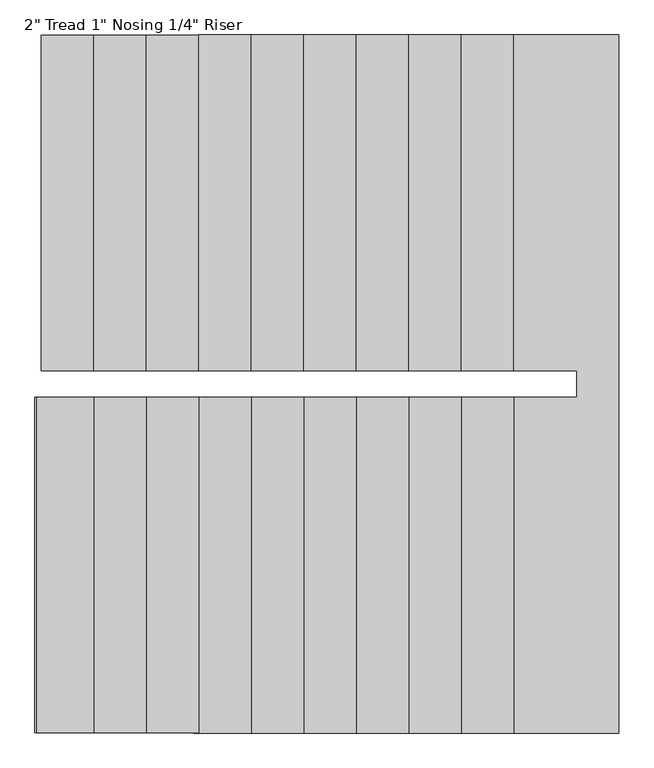
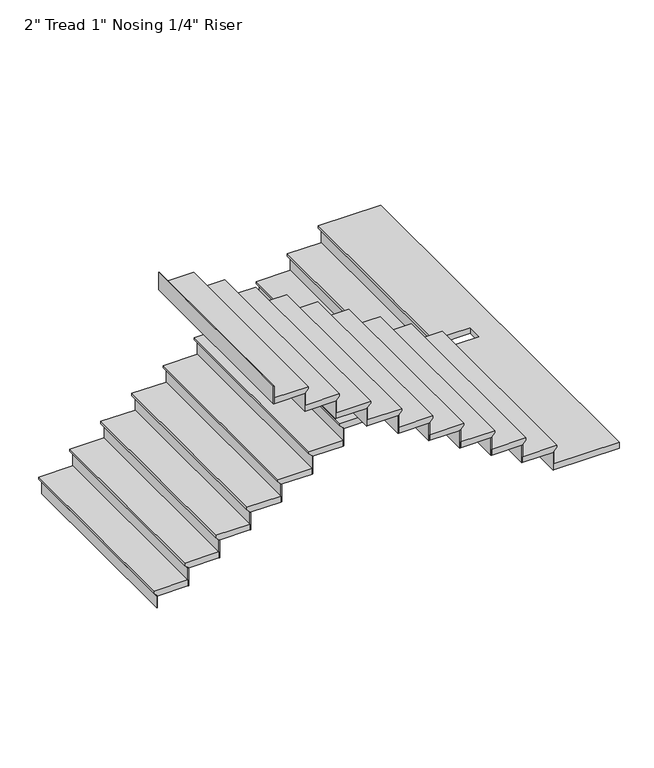
"""IFC4 building model written with IfcOpenShell, lengths in millimetres: stair flight geometry."""

from ifc_helpers import new_model, si_unit, origin, place, context, project, spatial, faceted_brep, source, transform, mapped, element, save


def stair_flight_de280899(model_context):
    return source(origin(), model_context, "Body", "Brep", [
        faceted_brep([(-6414.1711241, 10106.9344295, 3181.35), (-6414.1711241, 10106.9344295, 3200.4), (-6414.1711241, 11732.5344295, 3200.4), (-6414.1711241, 11732.5344295, 3181.35), (-6388.7711241, 10106.9344295, 3155.95), (-6388.7711241, 11732.5344295, 3155.95), (-6134.7711241, 10106.9344295, 3200.4), (-6134.7711241, 11732.5344295, 3200.4), (-6388.7711241, 11732.5344295, 3149.6), (-6134.7711241, 11732.5344295, 3149.6), (-6134.7711241, 10106.9344295, 3149.6), (-6388.7711241, 10106.9344295, 3149.6)], [[[0, 1, 2, 3]], [[4, 0, 3, 5]], [[2, 1, 6, 7]], [[8, 9, 10, 11]], [[2, 7, 9, 8, 5, 3]], [[8, 11, 4, 5]], [[6, 1, 0, 4, 11, 10]], [[7, 6, 10, 9]]]),
        faceted_brep([(-6388.7711241, 10106.9344295, 3149.6), (-6388.7711241, 10106.9344295, 3048.0), (-6382.4211241, 10106.9344295, 3048.0), (-6382.4211241, 10106.9344295, 3149.6), (-6388.7711241, 11732.5344295, 3149.6), (-6382.4211241, 11732.5344295, 3149.6), (-6382.4211241, 11732.5344295, 3048.0), (-6388.7711241, 11732.5344295, 3048.0)], [[[0, 1, 2, 3]], [[4, 5, 6, 7]], [[1, 0, 4, 7]], [[2, 1, 7, 6]], [[3, 2, 6, 5]], [[0, 3, 5, 4]]]),
        faceted_brep([(-6134.7711241, 10106.9344295, 3302.0), (-6134.7711241, 10106.9344295, 3149.6), (-6128.4211241, 10106.9344295, 3149.6), (-6128.4211241, 10106.9344295, 3302.0), (-6134.7711241, 11732.5344295, 3302.0), (-6128.4211241, 11732.5344295, 3302.0), (-6128.4211241, 11732.5344295, 3149.6), (-6134.7711241, 11732.5344295, 3149.6)], [[[0, 1, 2, 3]], [[4, 5, 6, 7]], [[1, 0, 4, 7]], [[2, 1, 7, 6]], [[3, 2, 6, 5]], [[0, 3, 5, 4]]]),
        faceted_brep([(-6160.1711241, 11732.5344295, 3352.8), (-6160.1711241, 10106.9344295, 3352.8), (-5880.7711241, 10106.9344295, 3352.8), (-5880.7711241, 11732.5344295, 3352.8), (-6134.7711241, 11732.5344295, 3302.0), (-5880.7711241, 11732.5344295, 3302.0), (-5880.7711241, 10106.9344295, 3302.0), (-6134.7711241, 10106.9344295, 3302.0), (-6134.7711241, 11732.5344295, 3308.35), (-6160.1711241, 11732.5344295, 3333.75), (-6134.7711241, 10106.9344295, 3308.35), (-6160.1711241, 10106.9344295, 3333.75)], [[[0, 1, 2, 3]], [[4, 5, 6, 7]], [[0, 3, 5, 4, 8, 9]], [[4, 7, 10, 8]], [[2, 1, 11, 10, 7, 6]], [[3, 2, 6, 5]], [[11, 1, 0, 9]], [[10, 11, 9, 8]]]),
        faceted_brep([(-5880.7711241, 10106.9344295, 3454.4), (-5880.7711241, 10106.9344295, 3302.0), (-5874.4211241, 10106.9344295, 3302.0), (-5874.4211241, 10106.9344295, 3454.4), (-5880.7711241, 11732.5344295, 3454.4), (-5874.4211241, 11732.5344295, 3454.4), (-5874.4211241, 11732.5344295, 3302.0), (-5880.7711241, 11732.5344295, 3302.0)], [[[0, 1, 2, 3]], [[4, 5, 6, 7]], [[1, 0, 4, 7]], [[2, 1, 7, 6]], [[3, 2, 6, 5]], [[0, 3, 5, 4]]]),
        faceted_brep([(-5906.1711241, 11732.5344295, 3505.2), (-5906.1711241, 10106.9344295, 3505.2), (-5626.7711241, 10106.9344295, 3505.2), (-5626.7711241, 11732.5344295, 3505.2), (-5880.7711241, 11732.5344295, 3454.4), (-5626.7711241, 11732.5344295, 3454.4), (-5626.7711241, 10106.9344295, 3454.4), (-5880.7711241, 10106.9344295, 3454.4), (-5880.7711241, 11732.5344295, 3460.75), (-5906.1711241, 11732.5344295, 3486.15), (-5880.7711241, 10106.9344295, 3460.75), (-5906.1711241, 10106.9344295, 3486.15)], [[[0, 1, 2, 3]], [[4, 5, 6, 7]], [[0, 3, 5, 4, 8, 9]], [[4, 7, 10, 8]], [[2, 1, 11, 10, 7, 6]], [[3, 2, 6, 5]], [[11, 1, 0, 9]], [[10, 11, 9, 8]]]),
        faceted_brep([(-5626.7711241, 10106.9344295, 3606.8), (-5626.7711241, 10106.9344295, 3454.4), (-5620.4211241, 10106.9344295, 3454.4), (-5620.4211241, 10106.9344295, 3606.8), (-5626.7711241, 11732.5344295, 3606.8), (-5620.4211241, 11732.5344295, 3606.8), (-5620.4211241, 11732.5344295, 3454.4), (-5626.7711241, 11732.5344295, 3454.4)], [[[0, 1, 2, 3]], [[4, 5, 6, 7]], [[1, 0, 4, 7]], [[2, 1, 7, 6]], [[3, 2, 6, 5]], [[0, 3, 5, 4]]]),
        faceted_brep([(-5652.1711241, 11732.5344295, 3657.6), (-5652.1711241, 10106.9344295, 3657.6), (-5372.7711241, 10106.9344295, 3657.6), (-5372.7711241, 11732.5344295, 3657.6), (-5626.7711241, 11732.5344295, 3606.8), (-5372.7711241, 11732.5344295, 3606.8), (-5372.7711241, 10106.9344295, 3606.8), (-5626.7711241, 10106.9344295, 3606.8), (-5626.7711241, 11732.5344295, 3613.15), (-5652.1711241, 11732.5344295, 3638.55), (-5626.7711241, 10106.9344295, 3613.15), (-5652.1711241, 10106.9344295, 3638.55)], [[[0, 1, 2, 3]], [[4, 5, 6, 7]], [[0, 3, 5, 4, 8, 9]], [[4, 7, 10, 8]], [[2, 1, 11, 10, 7, 6]], [[3, 2, 6, 5]], [[11, 1, 0, 9]], [[10, 11, 9, 8]]]),
        faceted_brep([(-5372.7711241, 10106.9344295, 3759.2), (-5372.7711241, 10106.9344295, 3606.8), (-5366.4211241, 10106.9344295, 3606.8), (-5366.4211241, 10106.9344295, 3759.2), (-5372.7711241, 11732.5344295, 3759.2), (-5366.4211241, 11732.5344295, 3759.2), (-5366.4211241, 11732.5344295, 3606.8), (-5372.7711241, 11732.5344295, 3606.8)], [[[0, 1, 2, 3]], [[4, 5, 6, 7]], [[1, 0, 4, 7]], [[2, 1, 7, 6]], [[3, 2, 6, 5]], [[0, 3, 5, 4]]]),
        faceted_brep([(-5398.1711241, 11732.5344295, 3810.0), (-5398.1711241, 10106.9344295, 3810.0), (-5118.7711241, 10106.9344295, 3810.0), (-5118.7711241, 11732.5344295, 3810.0), (-5372.7711241, 11732.5344295, 3759.2), (-5118.7711241, 11732.5344295, 3759.2), (-5118.7711241, 10106.9344295, 3759.2), (-5372.7711241, 10106.9344295, 3759.2), (-5372.7711241, 11732.5344295, 3765.55), (-5398.1711241, 11732.5344295, 3790.95), (-5372.7711241, 10106.9344295, 3765.55), (-5398.1711241, 10106.9344295, 3790.95)], [[[0, 1, 2, 3]], [[4, 5, 6, 7]], [[0, 3, 5, 4, 8, 9]], [[4, 7, 10, 8]], [[2, 1, 11, 10, 7, 6]], [[3, 2, 6, 5]], [[11, 1, 0, 9]], [[10, 11, 9, 8]]]),
        faceted_brep([(-5118.7711241, 10106.9344295, 3911.6), (-5118.7711241, 10106.9344295, 3759.2), (-5112.4211241, 10106.9344295, 3759.2), (-5112.4211241, 10106.9344295, 3911.6), (-5118.7711241, 11732.5344295, 3911.6), (-5112.4211241, 11732.5344295, 3911.6), (-5112.4211241, 11732.5344295, 3759.2), (-5118.7711241, 11732.5344295, 3759.2)], [[[0, 1, 2, 3]], [[4, 5, 6, 7]], [[1, 0, 4, 7]], [[2, 1, 7, 6]], [[3, 2, 6, 5]], [[0, 3, 5, 4]]]),
        faceted_brep([(-5144.1711241, 11732.5344295, 3962.4), (-5144.1711241, 10106.9344295, 3962.4), (-4864.7711241, 10106.9344295, 3962.4), (-4864.7711241, 11732.5344295, 3962.4), (-5118.7711241, 11732.5344295, 3911.6), (-4864.7711241, 11732.5344295, 3911.6), (-4864.7711241, 10106.9344295, 3911.6), (-5118.7711241, 10106.9344295, 3911.6), (-5118.7711241, 11732.5344295, 3917.95), (-5144.1711241, 11732.5344295, 3943.35), (-5118.7711241, 10106.9344295, 3917.95), (-5144.1711241, 10106.9344295, 3943.35)], [[[0, 1, 2, 3]], [[4, 5, 6, 7]], [[0, 3, 5, 4, 8, 9]], [[4, 7, 10, 8]], [[2, 1, 11, 10, 7, 6]], [[3, 2, 6, 5]], [[11, 1, 0, 9]], [[10, 11, 9, 8]]]),
        faceted_brep([(-4864.7711241, 10106.9344295, 4064.0), (-4864.7711241, 10106.9344295, 3911.6), (-4858.4211241, 10106.9344295, 3911.6), (-4858.4211241, 10106.9344295, 4064.0), (-4864.7711241, 11732.5344295, 4064.0), (-4858.4211241, 11732.5344295, 4064.0), (-4858.4211241, 11732.5344295, 3911.6), (-4864.7711241, 11732.5344295, 3911.6)], [[[0, 1, 2, 3]], [[4, 5, 6, 7]], [[1, 0, 4, 7]], [[2, 1, 7, 6]], [[3, 2, 6, 5]], [[0, 3, 5, 4]]]),
        faceted_brep([(-4890.1711241, 11732.5344295, 4114.8), (-4890.1711241, 10106.9344295, 4114.8), (-4610.7711241, 10106.9344295, 4114.8), (-4610.7711241, 11732.5344295, 4114.8), (-4864.7711241, 11732.5344295, 4064.0), (-4610.7711241, 11732.5344295, 4064.0), (-4610.7711241, 10106.9344295, 4064.0), (-4864.7711241, 10106.9344295, 4064.0), (-4864.7711241, 11732.5344295, 4070.35), (-4890.1711241, 11732.5344295, 4095.75), (-4864.7711241, 10106.9344295, 4070.35), (-4890.1711241, 10106.9344295, 4095.75)], [[[0, 1, 2, 3]], [[4, 5, 6, 7]], [[0, 3, 5, 4, 8, 9]], [[4, 7, 10, 8]], [[2, 1, 11, 10, 7, 6]], [[3, 2, 6, 5]], [[11, 1, 0, 9]], [[10, 11, 9, 8]]]),
        faceted_brep([(-4610.7711241, 10106.9344295, 4216.4), (-4610.7711241, 10106.9344295, 4064.0), (-4604.4211241, 10106.9344295, 4064.0), (-4604.4211241, 10106.9344295, 4216.4), (-4610.7711241, 11732.5344295, 4216.4), (-4604.4211241, 11732.5344295, 4216.4), (-4604.4211241, 11732.5344295, 4064.0), (-4610.7711241, 11732.5344295, 4064.0)], [[[0, 1, 2, 3]], [[4, 5, 6, 7]], [[1, 0, 4, 7]], [[2, 1, 7, 6]], [[3, 2, 6, 5]], [[0, 3, 5, 4]]]),
        faceted_brep([(-4636.1711241, 11732.5344295, 4267.2), (-4636.1711241, 10106.9344295, 4267.2), (-4356.7711241, 10106.9344295, 4267.2), (-4356.7711241, 11732.5344295, 4267.2), (-4610.7711241, 11732.5344295, 4216.4), (-4356.7711241, 11732.5344295, 4216.4), (-4356.7711241, 10106.9344295, 4216.4), (-4610.7711241, 10106.9344295, 4216.4), (-4610.7711241, 11732.5344295, 4222.75), (-4636.1711241, 11732.5344295, 4248.15), (-4610.7711241, 10106.9344295, 4222.75), (-4636.1711241, 10106.9344295, 4248.15)], [[[0, 1, 2, 3]], [[4, 5, 6, 7]], [[0, 3, 5, 4, 8, 9]], [[4, 7, 10, 8]], [[2, 1, 11, 10, 7, 6]], [[3, 2, 6, 5]], [[11, 1, 0, 9]], [[10, 11, 9, 8]]]),
        faceted_brep([(-4356.7711241, 10106.9344295, 4368.8), (-4356.7711241, 10106.9344295, 4216.4), (-4350.4211241, 10106.9344295, 4216.4), (-4350.4211241, 10106.9344295, 4368.8), (-4356.7711241, 11732.5344295, 4368.8), (-4350.4211241, 11732.5344295, 4368.8), (-4350.4211241, 11732.5344295, 4216.4), (-4356.7711241, 11732.5344295, 4216.4)], [[[0, 1, 2, 3]], [[4, 5, 6, 7]], [[1, 0, 4, 7]], [[2, 1, 7, 6]], [[3, 2, 6, 5]], [[0, 3, 5, 4]]]),
        faceted_brep([(-4382.1711241, 11732.5344295, 4419.6), (-4382.1711241, 10106.9344295, 4419.6), (-4102.7711241, 10106.9344295, 4419.6), (-4102.7711241, 11732.5344295, 4419.6), (-4356.7711241, 11732.5344295, 4368.8), (-4102.7711241, 11732.5344295, 4368.8), (-4102.7711241, 10106.9344295, 4368.8), (-4356.7711241, 10106.9344295, 4368.8), (-4356.7711241, 11732.5344295, 4375.15), (-4382.1711241, 11732.5344295, 4400.55), (-4356.7711241, 10106.9344295, 4375.15), (-4382.1711241, 10106.9344295, 4400.55)], [[[0, 1, 2, 3]], [[4, 5, 6, 7]], [[0, 3, 5, 4, 8, 9]], [[4, 7, 10, 8]], [[2, 1, 11, 10, 7, 6]], [[3, 2, 6, 5]], [[11, 1, 0, 9]], [[10, 11, 9, 8]]]),
        faceted_brep([(-4102.7711241, 10106.9344295, 4521.2), (-4102.7711241, 10106.9344295, 4368.8), (-4096.4211241, 10106.9344295, 4368.8), (-4096.4211241, 10106.9344295, 4521.2), (-4102.7711241, 11732.5344295, 4521.2), (-4096.4211241, 11732.5344295, 4521.2), (-4096.4211241, 11732.5344295, 4368.8), (-4102.7711241, 11732.5344295, 4368.8)], [[[0, 1, 2, 3]], [[4, 5, 6, 7]], [[1, 0, 4, 7]], [[2, 1, 7, 6]], [[3, 2, 6, 5]], [[0, 3, 5, 4]]]),
        faceted_brep([(-4153.5711241, 8354.3344295, 4572.0), (-3620.1711241, 8354.3344295, 4572.0), (-3620.1711241, 11732.5344295, 4572.0), (-4128.1711241, 11732.5344295, 4572.0), (-4128.1711241, 10106.9344295, 4572.0), (-3823.3711241, 10106.9344295, 4572.0), (-3823.3711241, 9979.9344295, 4572.0), (-4153.5711241, 9979.9344295, 4572.0), (-3620.1711241, 8354.3344295, 4521.2), (-4153.5711241, 8354.3344295, 4521.2), (-4153.5711241, 9979.9344295, 4521.2), (-3823.3711241, 9979.9344295, 4521.2), (-3823.3711241, 10106.9344295, 4521.2), (-4102.7711241, 10106.9344295, 4521.2), (-4102.7711241, 11732.5344295, 4521.2), (-3620.1711241, 11732.5344295, 4521.2), (-4102.7711241, 11732.5344295, 4527.55), (-4128.1711241, 11732.5344295, 4552.95), (-4102.7711241, 10106.9344295, 4527.55), (-4128.1711241, 10106.9344295, 4552.95)], [[[0, 1, 2, 3, 4, 5, 6, 7]], [[8, 9, 10, 11, 12, 13, 14, 15]], [[1, 0, 9, 8]], [[2, 1, 8, 15]], [[3, 2, 15, 14, 16, 17]], [[14, 13, 18, 16]], [[5, 4, 19, 18, 13, 12]], [[6, 5, 12, 11]], [[7, 6, 11, 10]], [[0, 7, 10, 9]], [[19, 4, 3, 17]], [[18, 19, 17, 16]]]),
        faceted_brep([(-4153.5711241, 9979.9344295, 4673.6), (-4153.5711241, 9979.9344295, 4521.2), (-4159.9211241, 9979.9344295, 4521.2), (-4159.9211241, 9979.9344295, 4673.6), (-4153.5711241, 8354.3344295, 4673.6), (-4159.9211241, 8354.3344295, 4673.6), (-4159.9211241, 8354.3344295, 4521.2), (-4153.5711241, 8354.3344295, 4521.2)], [[[0, 1, 2, 3]], [[4, 5, 6, 7]], [[1, 0, 4, 7]], [[2, 1, 7, 6]], [[3, 2, 6, 5]], [[0, 3, 5, 4]]]),
        faceted_brep([(-4128.1711241, 8354.3344295, 4724.4), (-4128.1711241, 9979.9344295, 4724.4), (-4407.5711241, 9979.9344295, 4724.4), (-4407.5711241, 8354.3344295, 4724.4), (-4153.5711241, 8354.3344295, 4673.6), (-4407.5711241, 8354.3344295, 4673.6), (-4407.5711241, 9979.9344295, 4673.6), (-4153.5711241, 9979.9344295, 4673.6), (-4153.5711241, 8354.3344295, 4679.95), (-4128.1711241, 8354.3344295, 4705.35), (-4153.5711241, 9979.9344295, 4679.95), (-4128.1711241, 9979.9344295, 4705.35)], [[[0, 1, 2, 3]], [[4, 5, 6, 7]], [[0, 3, 5, 4, 8, 9]], [[4, 7, 10, 8]], [[2, 1, 11, 10, 7, 6]], [[3, 2, 6, 5]], [[11, 1, 0, 9]], [[10, 11, 9, 8]]]),
        faceted_brep([(-4407.5711241, 9979.9344295, 4826.0), (-4407.5711241, 9979.9344295, 4673.6), (-4413.9211241, 9979.9344295, 4673.6), (-4413.9211241, 9979.9344295, 4826.0), (-4407.5711241, 8354.3344295, 4826.0), (-4413.9211241, 8354.3344295, 4826.0), (-4413.9211241, 8354.3344295, 4673.6), (-4407.5711241, 8354.3344295, 4673.6)], [[[0, 1, 2, 3]], [[4, 5, 6, 7]], [[1, 0, 4, 7]], [[2, 1, 7, 6]], [[3, 2, 6, 5]], [[0, 3, 5, 4]]]),
        faceted_brep([(-4382.1711241, 8354.3344295, 4876.8), (-4382.1711241, 9979.9344295, 4876.8), (-4661.5711241, 9979.9344295, 4876.8), (-4661.5711241, 8354.3344295, 4876.8), (-4407.5711241, 8354.3344295, 4826.0), (-4661.5711241, 8354.3344295, 4826.0), (-4661.5711241, 9979.9344295, 4826.0), (-4407.5711241, 9979.9344295, 4826.0), (-4407.5711241, 8354.3344295, 4832.35), (-4382.1711241, 8354.3344295, 4857.75), (-4407.5711241, 9979.9344295, 4832.35), (-4382.1711241, 9979.9344295, 4857.75)], [[[0, 1, 2, 3]], [[4, 5, 6, 7]], [[0, 3, 5, 4, 8, 9]], [[4, 7, 10, 8]], [[2, 1, 11, 10, 7, 6]], [[3, 2, 6, 5]], [[11, 1, 0, 9]], [[10, 11, 9, 8]]]),
        faceted_brep([(-4661.5711241, 9979.9344295, 4978.4), (-4661.5711241, 9979.9344295, 4826.0), (-4667.9211241, 9979.9344295, 4826.0), (-4667.9211241, 9979.9344295, 4978.4), (-4661.5711241, 8354.3344295, 4978.4), (-4667.9211241, 8354.3344295, 4978.4), (-4667.9211241, 8354.3344295, 4826.0), (-4661.5711241, 8354.3344295, 4826.0)], [[[0, 1, 2, 3]], [[4, 5, 6, 7]], [[1, 0, 4, 7]], [[2, 1, 7, 6]], [[3, 2, 6, 5]], [[0, 3, 5, 4]]]),
        faceted_brep([(-4636.1711241, 8354.3344295, 5029.2), (-4636.1711241, 9979.9344295, 5029.2), (-4915.5711241, 9979.9344295, 5029.2), (-4915.5711241, 8354.3344295, 5029.2), (-4661.5711241, 8354.3344295, 4978.4), (-4915.5711241, 8354.3344295, 4978.4), (-4915.5711241, 9979.9344295, 4978.4), (-4661.5711241, 9979.9344295, 4978.4), (-4661.5711241, 8354.3344295, 4984.75), (-4636.1711241, 8354.3344295, 5010.15), (-4661.5711241, 9979.9344295, 4984.75), (-4636.1711241, 9979.9344295, 5010.15)], [[[0, 1, 2, 3]], [[4, 5, 6, 7]], [[0, 3, 5, 4, 8, 9]], [[4, 7, 10, 8]], [[2, 1, 11, 10, 7, 6]], [[3, 2, 6, 5]], [[11, 1, 0, 9]], [[10, 11, 9, 8]]]),
        faceted_brep([(-4915.5711241, 9979.9344295, 5130.8), (-4915.5711241, 9979.9344295, 4978.4), (-4921.9211241, 9979.9344295, 4978.4), (-4921.9211241, 9979.9344295, 5130.8), (-4915.5711241, 8354.3344295, 5130.8), (-4921.9211241, 8354.3344295, 5130.8), (-4921.9211241, 8354.3344295, 4978.4), (-4915.5711241, 8354.3344295, 4978.4)], [[[0, 1, 2, 3]], [[4, 5, 6, 7]], [[1, 0, 4, 7]], [[2, 1, 7, 6]], [[3, 2, 6, 5]], [[0, 3, 5, 4]]]),
        faceted_brep([(-4890.1711241, 8354.3344295, 5181.6), (-4890.1711241, 9979.9344295, 5181.6), (-5169.5711241, 9979.9344295, 5181.6), (-5169.5711241, 8354.3344295, 5181.6), (-4915.5711241, 8354.3344295, 5130.8), (-5169.5711241, 8354.3344295, 5130.8), (-5169.5711241, 9979.9344295, 5130.8), (-4915.5711241, 9979.9344295, 5130.8), (-4915.5711241, 8354.3344295, 5137.15), (-4890.1711241, 8354.3344295, 5162.55), (-4915.5711241, 9979.9344295, 5137.15), (-4890.1711241, 9979.9344295, 5162.55)], [[[0, 1, 2, 3]], [[4, 5, 6, 7]], [[0, 3, 5, 4, 8, 9]], [[4, 7, 10, 8]], [[2, 1, 11, 10, 7, 6]], [[3, 2, 6, 5]], [[11, 1, 0, 9]], [[10, 11, 9, 8]]]),
        faceted_brep([(-5169.5711241, 9979.9344295, 5283.2), (-5169.5711241, 9979.9344295, 5130.8), (-5175.9211241, 9979.9344295, 5130.8), (-5175.9211241, 9979.9344295, 5283.2), (-5169.5711241, 8354.3344295, 5283.2), (-5175.9211241, 8354.3344295, 5283.2), (-5175.9211241, 8354.3344295, 5130.8), (-5169.5711241, 8354.3344295, 5130.8)], [[[0, 1, 2, 3]], [[4, 5, 6, 7]], [[1, 0, 4, 7]], [[2, 1, 7, 6]], [[3, 2, 6, 5]], [[0, 3, 5, 4]]]),
        faceted_brep([(-5144.1711241, 8354.3344295, 5334.0), (-5144.1711241, 9979.9344295, 5334.0), (-5423.5711241, 9979.9344295, 5334.0), (-5423.5711241, 8354.3344295, 5334.0), (-5169.5711241, 8354.3344295, 5283.2), (-5423.5711241, 8354.3344295, 5283.2), (-5423.5711241, 9979.9344295, 5283.2), (-5169.5711241, 9979.9344295, 5283.2), (-5169.5711241, 8354.3344295, 5289.55), (-5144.1711241, 8354.3344295, 5314.95), (-5169.5711241, 9979.9344295, 5289.55), (-5144.1711241, 9979.9344295, 5314.95)], [[[0, 1, 2, 3]], [[4, 5, 6, 7]], [[0, 3, 5, 4, 8, 9]], [[4, 7, 10, 8]], [[2, 1, 11, 10, 7, 6]], [[3, 2, 6, 5]], [[11, 1, 0, 9]], [[10, 11, 9, 8]]]),
        faceted_brep([(-5423.5711241, 9979.9344295, 5435.6), (-5423.5711241, 9979.9344295, 5283.2), (-5429.9211241, 9979.9344295, 5283.2), (-5429.9211241, 9979.9344295, 5435.6), (-5423.5711241, 8354.3344295, 5435.6), (-5429.9211241, 8354.3344295, 5435.6), (-5429.9211241, 8354.3344295, 5283.2), (-5423.5711241, 8354.3344295, 5283.2)], [[[0, 1, 2, 3]], [[4, 5, 6, 7]], [[1, 0, 4, 7]], [[2, 1, 7, 6]], [[3, 2, 6, 5]], [[0, 3, 5, 4]]]),
        faceted_brep([(-5398.1711241, 8354.3344295, 5486.4), (-5398.1711241, 9979.9344295, 5486.4), (-5677.5711241, 9979.9344295, 5486.4), (-5677.5711241, 8354.3344295, 5486.4), (-5423.5711241, 8354.3344295, 5435.6), (-5677.5711241, 8354.3344295, 5435.6), (-5677.5711241, 9979.9344295, 5435.6), (-5423.5711241, 9979.9344295, 5435.6), (-5423.5711241, 8354.3344295, 5441.95), (-5398.1711241, 8354.3344295, 5467.35), (-5423.5711241, 9979.9344295, 5441.95), (-5398.1711241, 9979.9344295, 5467.35)], [[[0, 1, 2, 3]], [[4, 5, 6, 7]], [[0, 3, 5, 4, 8, 9]], [[4, 7, 10, 8]], [[2, 1, 11, 10, 7, 6]], [[3, 2, 6, 5]], [[11, 1, 0, 9]], [[10, 11, 9, 8]]]),
        faceted_brep([(-5677.5711241, 9979.9344295, 5588.0), (-5677.5711241, 9979.9344295, 5435.6), (-5683.9211241, 9979.9344295, 5435.6), (-5683.9211241, 9979.9344295, 5588.0), (-5677.5711241, 8354.3344295, 5588.0), (-5683.9211241, 8354.3344295, 5588.0), (-5683.9211241, 8354.3344295, 5435.6), (-5677.5711241, 8354.3344295, 5435.6)], [[[0, 1, 2, 3]], [[4, 5, 6, 7]], [[1, 0, 4, 7]], [[2, 1, 7, 6]], [[3, 2, 6, 5]], [[0, 3, 5, 4]]]),
        faceted_brep([(-5652.1711241, 8354.3344295, 5638.8), (-5652.1711241, 9979.9344295, 5638.8), (-5931.5711241, 9979.9344295, 5638.8), (-5931.5711241, 8354.3344295, 5638.8), (-5677.5711241, 8354.3344295, 5588.0), (-5931.5711241, 8354.3344295, 5588.0), (-5931.5711241, 9979.9344295, 5588.0), (-5677.5711241, 9979.9344295, 5588.0), (-5677.5711241, 8354.3344295, 5594.35), (-5652.1711241, 8354.3344295, 5619.75), (-5677.5711241, 9979.9344295, 5594.35), (-5652.1711241, 9979.9344295, 5619.75)], [[[0, 1, 2, 3]], [[4, 5, 6, 7]], [[0, 3, 5, 4, 8, 9]], [[4, 7, 10, 8]], [[2, 1, 11, 10, 7, 6]], [[3, 2, 6, 5]], [[11, 1, 0, 9]], [[10, 11, 9, 8]]]),
        faceted_brep([(-5931.5711241, 9979.9344295, 5740.4), (-5931.5711241, 9979.9344295, 5588.0), (-5937.9211241, 9979.9344295, 5588.0), (-5937.9211241, 9979.9344295, 5740.4), (-5931.5711241, 8354.3344295, 5740.4), (-5937.9211241, 8354.3344295, 5740.4), (-5937.9211241, 8354.3344295, 5588.0), (-5931.5711241, 8354.3344295, 5588.0)], [[[0, 1, 2, 3]], [[4, 5, 6, 7]], [[1, 0, 4, 7]], [[2, 1, 7, 6]], [[3, 2, 6, 5]], [[0, 3, 5, 4]]]),
        faceted_brep([(-5906.1711241, 8354.3344295, 5791.2), (-5906.1711241, 9979.9344295, 5791.2), (-6185.5711241, 9979.9344295, 5791.2), (-6185.5711241, 8354.3344295, 5791.2), (-5931.5711241, 8354.3344295, 5740.4), (-6185.5711241, 8354.3344295, 5740.4), (-6185.5711241, 9979.9344295, 5740.4), (-5931.5711241, 9979.9344295, 5740.4), (-5931.5711241, 8354.3344295, 5746.75), (-5906.1711241, 8354.3344295, 5772.15), (-5931.5711241, 9979.9344295, 5746.75), (-5906.1711241, 9979.9344295, 5772.15)], [[[0, 1, 2, 3]], [[4, 5, 6, 7]], [[0, 3, 5, 4, 8, 9]], [[4, 7, 10, 8]], [[2, 1, 11, 10, 7, 6]], [[3, 2, 6, 5]], [[11, 1, 0, 9]], [[10, 11, 9, 8]]]),
        faceted_brep([(-6185.5711241, 9979.9344295, 5892.8), (-6185.5711241, 9979.9344295, 5740.4), (-6191.9211241, 9979.9344295, 5740.4), (-6191.9211241, 9979.9344295, 5892.8), (-6185.5711241, 8354.3344295, 5892.8), (-6191.9211241, 8354.3344295, 5892.8), (-6191.9211241, 8354.3344295, 5740.4), (-6185.5711241, 8354.3344295, 5740.4)], [[[0, 1, 2, 3]], [[4, 5, 6, 7]], [[1, 0, 4, 7]], [[2, 1, 7, 6]], [[3, 2, 6, 5]], [[0, 3, 5, 4]]]),
        faceted_brep([(-6439.5711241, 9979.9344295, 6045.2), (-6439.5711241, 9979.9344295, 5892.8), (-6445.9211241, 9979.9344295, 5892.8), (-6445.9211241, 9979.9344295, 6045.2), (-6439.5711241, 8354.3344295, 6045.2), (-6445.9211241, 8354.3344295, 6045.2), (-6445.9211241, 8354.3344295, 5892.8), (-6439.5711241, 8354.3344295, 5892.8)], [[[0, 1, 2, 3]], [[4, 5, 6, 7]], [[1, 0, 4, 7]], [[2, 1, 7, 6]], [[3, 2, 6, 5]], [[0, 3, 5, 4]]]),
        faceted_brep([(-6160.1711241, 8354.3344295, 5943.6), (-6160.1711241, 9979.9344295, 5943.6), (-6439.5711241, 9979.9344295, 5943.6), (-6439.5711241, 8354.3344295, 5943.6), (-6185.5711241, 8354.3344295, 5892.8), (-6439.5711241, 8354.3344295, 5892.8), (-6439.5711241, 9979.9344295, 5892.8), (-6185.5711241, 9979.9344295, 5892.8), (-6185.5711241, 8354.3344295, 5899.15), (-6160.1711241, 8354.3344295, 5924.55), (-6185.5711241, 9979.9344295, 5899.15), (-6160.1711241, 9979.9344295, 5924.55)], [[[0, 1, 2, 3]], [[4, 5, 6, 7]], [[0, 3, 5, 4, 8, 9]], [[4, 7, 10, 8]], [[2, 1, 11, 10, 7, 6]], [[3, 2, 6, 5]], [[11, 1, 0, 9]], [[10, 11, 9, 8]]]),
    ])


if __name__ == "__main__":
    model = new_model("IFC4")
    model_context = context("Model", 3, world=origin())
    ifc_project = project(units=[si_unit("LENGTHUNIT", "METRE", prefix="MILLI")], contexts=[model_context])
    site = spatial("IfcSite", under=ifc_project)
    building = spatial("IfcBuilding", under=site)
    placement = place(None, origin())
    stair_flight_shape = stair_flight_de280899(model_context)
    element("IfcStairFlight", 1, ObjectType="2\" Tread 1\" Nosing 1/4\" Riser", at=placement, inside=building, context=model_context, shape_type="MappedRepresentation", body=[
        mapped(stair_flight_shape, transform((0.0, 0.0, 0.0), x_axis=(1.0, 0.0, 0.0), y_axis=(0.0, 1.0, 0.0), z_axis=(0.0, 0.0, 1.0))),
    ])
    save(model, "model.ifc")
